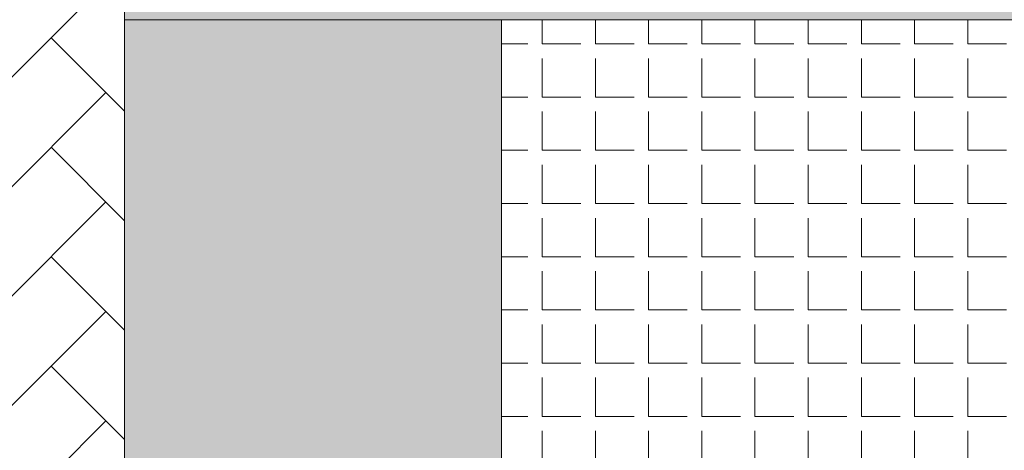
# Model space of a CAD drawing. Units: inches. Extents: x 84 to 1044, y -280 to 906.
# Tile 14 of 105: x 441 to 571, y -25 to 31. Entities that reach past the tile are written whole.
import ezdxf

# ---------------------------------------------------------------- set-up
doc = ezdxf.new("R2010")
doc.units = ezdxf.units.IN
for name, color, linetype, lineweight, true_color in [('A-FLOR-STRS-PATT', 35, 'Continuous', 9, 0x947764), ('L-HRDS-PATT', 23, 'Continuous', 9, 0xc2877b), ('L-PRKG-PATT', 35, 'Continuous', 9, 0x947764)]:
    doc.layers.add(name, color=color, linetype=linetype, lineweight=lineweight, true_color=true_color)
doc.layers.add('A-STAIRCASE', color=144, linetype='Continuous', lineweight=18)
doc.layers.add('L-HRDS', color=32, linetype='Continuous', lineweight=18)

msp = doc.modelspace()

# ---------------------------------------------------------------- hatches: boundary and pattern name
at = {"layer": 'A-FLOR-STRS-PATT', "transparency": 33554567}
h = msp.add_hatch(color=256, dxfattribs=at)
h.dxf.hatch_style = 1
h.paths.add_polyline_path([(650.074, 91.12), (638.074, 91.12), (638.074, 67.12), (455.074, 67.12), (455.074, 55.12), (650.074, 55.12)], flags=17)
h.paths.add_polyline_path([(662.074, 91.12), (650.074, 91.12), (650.074, 55.12), (455.074, 55.12), (455.074, 43.12), (662.074, 43.12)])
h.paths.add_polyline_path([(674.074, 91.12), (671.074, 91.12), (662.074, 91.12), (662.074, 43.12), (455.074, 43.12), (455.074, 31.12), (674.074, 31.12)])
h.paths.add_polyline_path([(227.179, 151.12), (203.179, 151.12), (143.179, 151.12), (143.179, 139.12), (227.179, 139.12)])
h.paths.add_polyline_path([(227.179, 139.12), (143.179, 139.12), (143.179, 127.12), (227.179, 127.12)])
h.paths.add_polyline_path([(203.179, 271.12), (143.179, 271.12), (143.179, 259.12), (203.179, 259.12)])
h.paths.add_polyline_path([(203.179, 259.12), (143.179, 259.12), (143.179, 247.12), (203.179, 247.12)])
h.paths.add_polyline_path([(203.179, 769.12), (143.179, 769.12), (143.179, 757.12), (203.179, 757.12)])
h.paths.add_polyline_path([(203.179, 757.12), (143.179, 757.12), (143.179, 745.12), (203.179, 745.12)])
h.paths.add_polyline_path([(434.074, 847.12), (422.074, 847.12), (422.074, 769.12), (434.074, 769.12)])
h.paths.add_polyline_path([(422.074, 847.12), (410.074, 847.12), (410.074, 769.12), (422.074, 769.12)])
at = {"layer": 'L-HRDS-PATT', "transparency": 33554567}
h = msp.add_hatch(color=256, dxfattribs=at)
h.dxf.hatch_style = 1
h.paths.add_polyline_path([(504.574, 31.12), (455.074, 31.12), (455.074, -40.88), (504.574, -40.88)])
h = msp.add_hatch(dxfattribs=at)
h.set_pattern_fill('ANGLE', color=256)
h.set_pattern_definition([(0, (0, 0), (0, 6.985), [5.08, -1.905]), (90, (0, 0), (-6.985, 4e-16), [5.08, -1.905])])
h.paths.add_polyline_path([(650.074, 31.12), (504.574, 31.12), (504.574, -112.88), (504.574, -121.88), (624.574, -121.88), (624.574, -112.88), (650.074, -112.88)])
at = {"layer": 'L-PRKG-PATT', "transparency": 33554567}
h = msp.add_hatch(dxfattribs=at)
h.set_pattern_fill('AR-HBONE', color=256, scale=0.1)
h.paths.add_polyline_path([(455.074, 31.12), (455.074, 91.12), (455.074, 151.12), (413.127, 151.12), (341.127, 151.12), (290.179, 151.12), (227.179, 151.12), (227.179, 127.12), (143.179, 127.12), (143.179, -112.88), (143.179, -117.88), (455.074, -117.88)])

# ---------------------------------------------------------------- linework, layer by layer
at = {"layer": 'A-STAIRCASE'}
msp.add_line((455.074, 91.12), (455.074, 31.12), dxfattribs=at)
msp.add_lwpolyline([(674.074, 91.12), (674.074, 31.12), (455.074, 31.12)], dxfattribs=at)
at = {"layer": 'L-HRDS'}
for p, q in [((455.074, 31.12), (455.074, -121.88)), ((504.574, -112.88), (504.574, 31.12))]:
    msp.add_line(p, q, dxfattribs=at)

doc.saveas('drawing.dxf')
